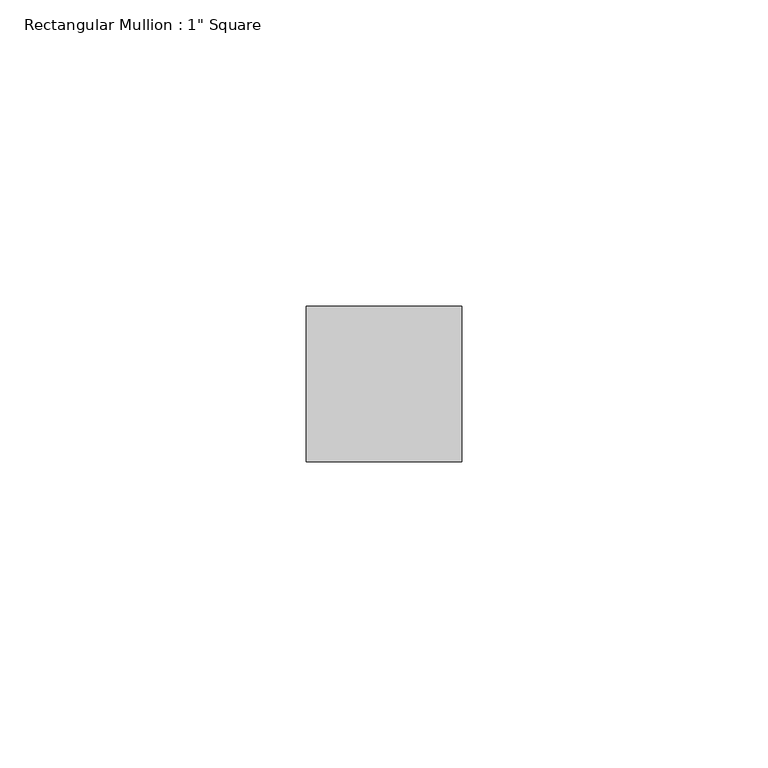
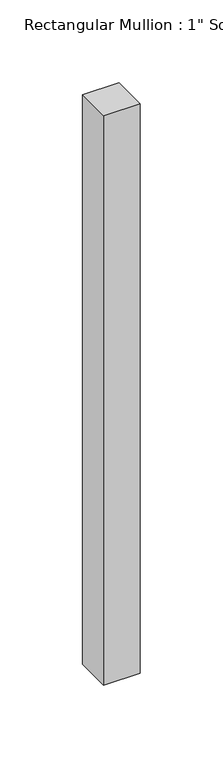
"""IFC4 building model written with IfcOpenShell, lengths in millimetres: member geometry."""

from ifc_helpers import new_model, si_unit, frame, origin, place, context, project, spatial, polyline, outline, extrude, source, transform, mapped, element, save


def member_ff98d70f(model_context):
    return source(origin(), model_context, "Body", "SweptSolid", [
        extrude(outline(polyline([(12.7, 12.7), (12.7, -12.7), (-12.7, -12.7), (-12.7, 12.7), (12.7, 12.7)])), frame((0.0, 0.0, -419.1), z_axis=(0.0, 0.0, 1.0), x_axis=(1.0, 0.0, 0.0)), (0.0, 0.0, 1.0), 419.1),
    ])


if __name__ == "__main__":
    model = new_model("IFC4")
    model_context = context("Model", 3, world=origin())
    ifc_project = project(units=[si_unit("LENGTHUNIT", "METRE", prefix="MILLI")], contexts=[model_context])
    site = spatial("IfcSite", under=ifc_project)
    building = spatial("IfcBuilding", under=site)
    placement = place(None, origin())
    member_shape = member_ff98d70f(model_context)
    element("IfcMember", 1, ObjectType="Rectangular Mullion : 1\" Square", at=placement, inside=building, context=model_context, shape_type="MappedRepresentation", body=[
        mapped(member_shape, transform((0.0, 0.0, 0.0), x_axis=(1.0, 0.0, 0.0), y_axis=(0.0, 1.0, 0.0), z_axis=(0.0, 0.0, 1.0))),
    ])
    save(model, "model.ifc")

# Revit data of these elements
# Type "Rectangular Mullion : 1\" Square"
#   built-in parameter 1007304 = 0.0833333 (stored number, unit not read)
#   built-in parameter 1007301 = 0.0416667 (stored number, unit not read)
#   built-in parameter 1007300 = 0.0416667 (stored number, unit not read)
# Element 1 (IfcMember, "Rectangular Mullion : 1\" Square")
#   Materials on its faces: "Aluminum"
# Materials
#   "Aluminum": class "Metal", colour RGB 247 247 247, transparency 0, Description = "Aluminum 6061", Cost = 0
